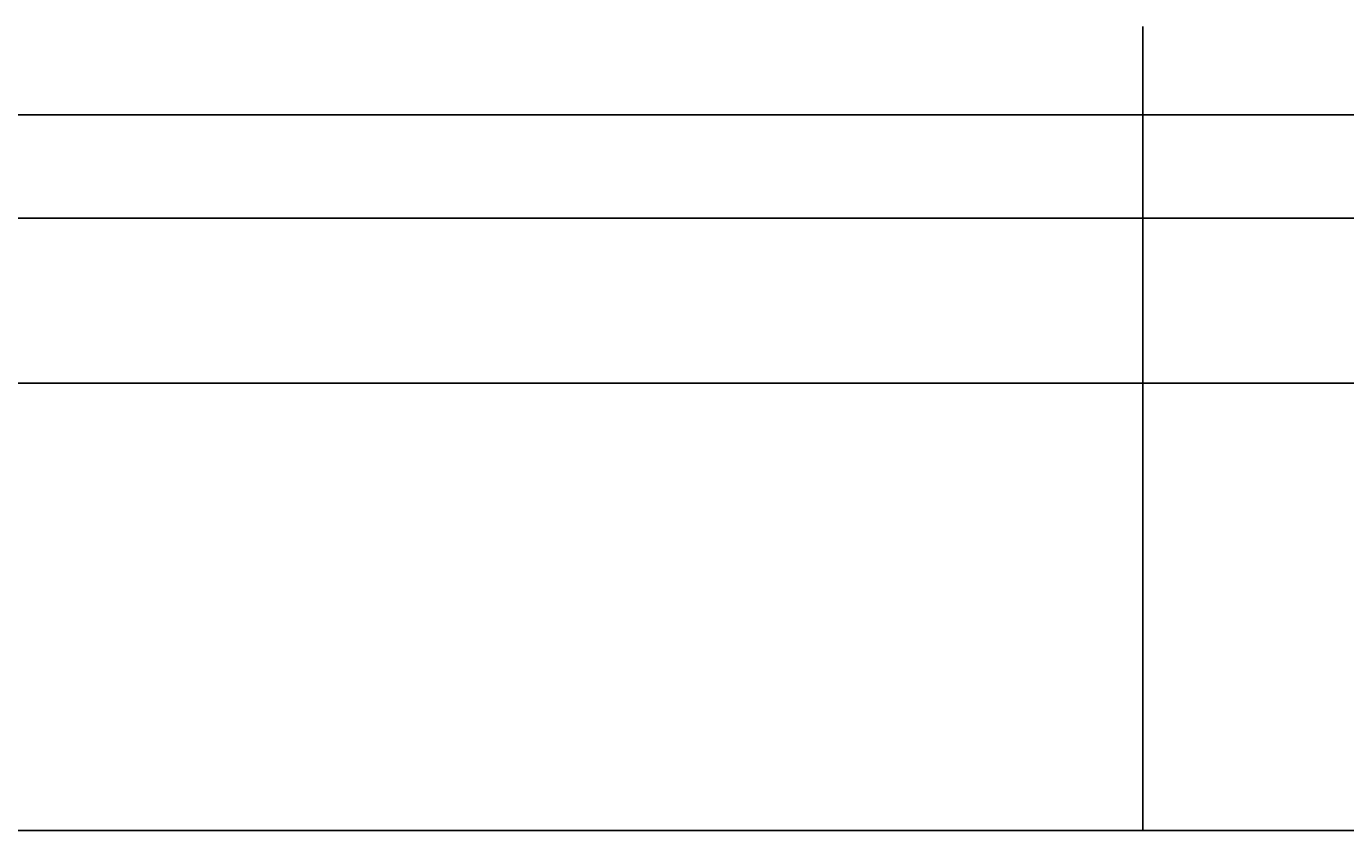
# Model space of a CAD drawing. Units: inches. Extents: x 35362 to 73946, y 43607 to 67532.
# Tile 7 of 134: x 40793 to 46225, y 43607 to 46919. Entities that reach past the tile are written whole.
import ezdxf

# ---------------------------------------------------------------- set-up
doc = ezdxf.new("R2010")
doc.units = ezdxf.units.IN
doc.header["$MEASUREMENT"] = 0
doc.layers.add('A-ANNO-DIMS', color=2, linetype='Continuous', lineweight=18)
doc.styles.get("Standard").update_dxf_attribs({"font": 'arial.ttf'})
doc.dimstyles.get("Standard").update_dxf_attribs({"dimtxt": 0.18, "dimasz": 0.18, "dimexe": 0.18, "dimexo": 0.0625, "dimgap": 0.09, "dimtad": 0, "dimtih": 1, "dimtoh": 1, "dimdec": 4, "dimzin": 0, "dimdsep": 46, "dimtxsty": 'Standard', "dimcen": 0.09, "dimadec": 0, "dimazin": 0, "dimtfac": 1, "dimtdec": 4, "dimtofl": 0, "dimtmove": 0, "dimatfit": 3, "dimfxl": 1, "dimtolj": 1, "dimtzin": 0, "dimarcsym": 0})

# ---------------------------------------------------------------- blocks, each defined once
blk = doc.blocks.new('*D5')
at = {"layer": 'A-ANNO-DIMS', "color": 0, "lineweight": -2, "transparency": 16777216}
for p, q in [((37121.9, 46919.3), (37121.9, 43606.7)), ((69871.5, 45449.8), (69871.5, 43606.7)), ((37122.1, 43606.9), (53496.3, 43606.9)), ((69871.3, 43606.9), (53497.2, 43606.9))]:
    blk.add_line(p, q, dxfattribs=at)
at = {"layer": 'A-ANNO-DIMS', "color": 0, "transparency": 16777216}
for points in [[(37122.1, 43606.9), (37122.1, 43606.8), (37121.9, 43606.9)], [(69871.3, 43606.9), (69871.3, 43606.8), (69871.5, 43606.9)]]:
    blk.add_solid(points, dxfattribs=at)
at = {"layer": 'Defpoints', "color": 0, "transparency": 16777216}
for p in [(37121.9, 46919.4), (69871.5, 45449.9), (69871.5, 43606.9)]:
    blk.add_point(p, dxfattribs=at)
at = {"layer": 'A-ANNO-DIMS', "color": 0, "transparency": 16777216, "insert": (53496.7, 43606.9), "char_height": 0.18, "attachment_point": 5}
blk.add_mtext('\\A1;32750', dxfattribs=at)
blk = doc.blocks.new('*D41')
at = {"layer": 'A-ANNO-DIMS', "color": 0, "lineweight": -2, "transparency": 16777216}
for p, q in [((39894.8, 46919.3), (39894.8, 43606.7)), ((45390.1, 46919.3), (45390.1, 43606.7)), ((39895, 43606.9), (42642, 43606.9)), ((45390, 43606.9), (42643, 43606.9))]:
    blk.add_line(p, q, dxfattribs=at)
at = {"layer": 'A-ANNO-DIMS', "color": 0, "transparency": 16777216}
for points in [[(39895, 43606.9), (39895, 43606.8), (39894.8, 43606.9)], [(45390, 43606.9), (45390, 43606.8), (45390.1, 43606.9)]]:
    blk.add_solid(points, dxfattribs=at)
at = {"layer": 'Defpoints', "color": 0, "transparency": 16777216}
for p in [(39894.8, 46919.4), (45390.1, 46919.4), (45390.1, 43606.9)]:
    blk.add_point(p, dxfattribs=at)
at = {"layer": 'A-ANNO-DIMS', "color": 0, "transparency": 16777216, "insert": (42642.5, 43606.9), "char_height": 0.18, "attachment_point": 5}
blk.add_mtext('\\A1;5495.3', dxfattribs=at)
blk = doc.blocks.new('*D67')
at = {"layer": 'A-ANNO-DIMS', "color": 0, "lineweight": -2, "transparency": 16777216}
for p, q in [((56873.5, 53351.5), (35361.8, 53351.5)), ((35361.9, 53351.3), (35361.9, 49400.9)), ((35361.9, 45450.1), (35361.9, 49400.5)), ((53793.6, 45449.9), (35361.8, 45449.9))]:
    blk.add_line(p, q, dxfattribs=at)
at = {"layer": 'A-ANNO-DIMS', "color": 0, "transparency": 16777216}
for points in [[(35361.9, 53351.3), (35362, 53351.3), (35361.9, 53351.5)], [(35361.9, 45450.1), (35362, 45450.1), (35361.9, 45449.9)]]:
    blk.add_solid(points, dxfattribs=at)
at = {"layer": 'Defpoints', "color": 0, "transparency": 16777216}
for p in [(35361.9, 53351.5), (56873.6, 53351.5), (53793.6, 45449.9)]:
    blk.add_point(p, dxfattribs=at)
at = {"layer": 'A-ANNO-DIMS', "color": 0, "transparency": 16777216, "insert": (35361.9, 49400.7), "char_height": 0.18, "attachment_point": 5}
blk.add_mtext('\\A1;7901.6', dxfattribs=at)
blk = doc.blocks.new('*D76')
at = {"layer": 'A-ANNO-DIMS', "color": 0, "lineweight": -2, "transparency": 16777216}
for p, q in [((54052.8, 46555.3), (35361.8, 46555.3)), ((35361.9, 46555.1), (35361.9, 46342.3)), ((35361.9, 46129.1), (35361.9, 46341.9)), ((53793.6, 46128.9), (35361.8, 46128.9))]:
    blk.add_line(p, q, dxfattribs=at)
at = {"layer": 'A-ANNO-DIMS', "color": 0, "transparency": 16777216}
for points in [[(35361.9, 46555.1), (35362, 46555.1), (35361.9, 46555.3)], [(35361.9, 46129.1), (35362, 46129.1), (35361.9, 46128.9)]]:
    blk.add_solid(points, dxfattribs=at)
at = {"layer": 'Defpoints', "color": 0, "transparency": 16777216}
for p in [(35361.9, 46555.3), (54052.9, 46555.3), (53793.6, 46128.9)]:
    blk.add_point(p, dxfattribs=at)
at = {"layer": 'A-ANNO-DIMS', "color": 0, "transparency": 16777216, "insert": (35361.9, 46342.1), "char_height": 0.18, "attachment_point": 5}
blk.add_mtext('\\A1;426.4', dxfattribs=at)
blk = doc.blocks.new('*D90')
at = {"layer": 'A-ANNO-DIMS', "color": 0, "lineweight": -2, "transparency": 16777216}
for p, q in [((53707.7, 47291.3), (35361.8, 47291.3)), ((35361.9, 47291.1), (35361.9, 46710.3)), ((35361.9, 46129.1), (35361.9, 46709.9)), ((53793.6, 46128.9), (35361.8, 46128.9))]:
    blk.add_line(p, q, dxfattribs=at)
at = {"layer": 'A-ANNO-DIMS', "color": 0, "transparency": 16777216}
for points in [[(35361.9, 47291.1), (35362, 47291.1), (35361.9, 47291.3)], [(35361.9, 46129.1), (35362, 46129.1), (35361.9, 46128.9)]]:
    blk.add_solid(points, dxfattribs=at)
at = {"layer": 'Defpoints', "color": 0, "transparency": 16777216}
for p in [(53707.8, 47291.3), (35361.9, 46128.9), (53793.6, 46128.9)]:
    blk.add_point(p, dxfattribs=at)
at = {"layer": 'A-ANNO-DIMS', "color": 0, "transparency": 16777216, "insert": (35361.9, 46710.1), "char_height": 0.18, "attachment_point": 5}
blk.add_mtext('\\A1;1162.4', dxfattribs=at)

msp = doc.modelspace()

# ---------------------------------------------------------------- dimensions: what is measured, and where the dimension line sits
at = {"layer": 'A-ANNO-DIMS'}
for base, p1, p2, picture, middle in [((35361.949, 53351.529), (53793.638, 45449.894), (56873.602, 53351.529), '*D67', (35361.949, 49400.712)), ((35361.949, 46128.878), (53707.781, 47291.285), (53793.638, 46128.878), '*D90', (35361.949, 46710.081)), ((35361.949, 46555.293), (53793.638, 46128.878), (54052.899, 46555.293), '*D76', (35361.949, 46342.086))]:
    dim = msp.add_linear_dim(base=base, p1=p1, p2=p2, angle=90, dimstyle='Standard', override={"dimdec": 1, "dimlfac": 1, "dimrnd": 0, "dimzin": 0, "dimdsep": 46, "dimlunit": 2}, dxfattribs=at)
    dim.commit()
    dim.dimension.update_dxf_attribs({"geometry": picture, "text_midpoint": middle})
for base, p1, p2, override, picture, middle in [((69871.496, 43606.859), (37121.949, 46919.381), (69871.496, 45449.894), {"dimdec": 0, "dimlfac": 1, "dimrnd": 0, "dimzin": 0, "dimdsep": 46, "dimlunit": 2}, '*D5', (53496.723, 43606.859)), ((45390.147, 43606.859), (39894.84, 46919.381), (45390.147, 46919.381), {"dimdec": 1, "dimlfac": 1, "dimrnd": 0, "dimzin": 0, "dimdsep": 46, "dimlunit": 2}, '*D41', (42642.494, 43606.859))]:
    dim = msp.add_linear_dim(base=base, p1=p1, p2=p2, dimstyle='Standard', override=override, dxfattribs=at)
    dim.commit()
    dim.dimension.update_dxf_attribs({"geometry": picture, "text_midpoint": middle})

doc.saveas('drawing.dxf')
